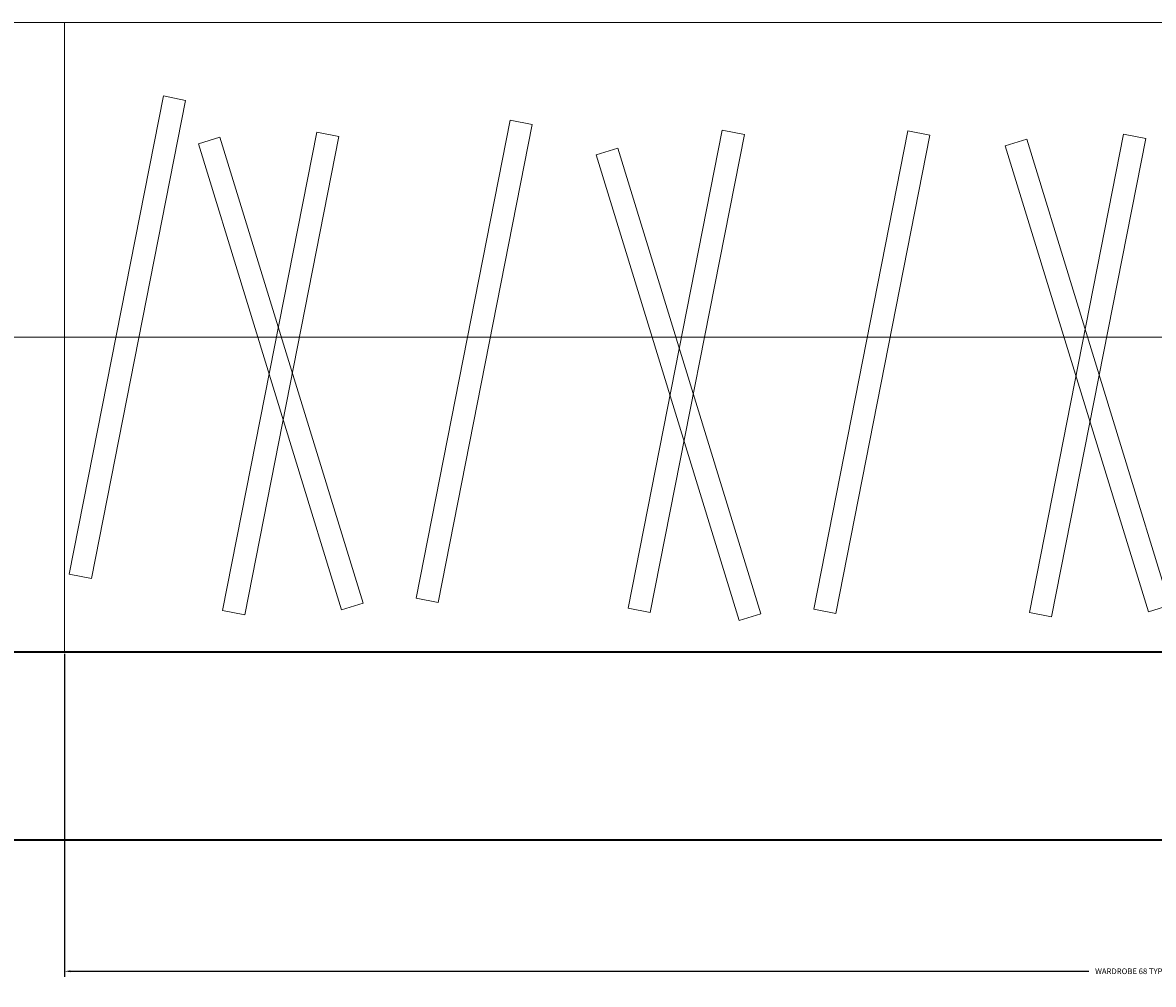
# Model space of a CAD drawing. Units: inches. Extents: x -61 to 1599, y -1316 to 257.
# Tile 180 of 204: x 1444 to 1480, y -788 to -757. Entities that reach past the tile are written whole.
import ezdxf

# ---------------------------------------------------------------- set-up
doc = ezdxf.new("R2010")
doc.units = ezdxf.units.IN
doc.header["$MEASUREMENT"] = 0
for name, color, linetype, lineweight in [('A-ANNO-DIMS', 2, 'Continuous', 18), ('A-FLOR-CASE', 8, 'Continuous', 18), ('WALLS', 4, 'Continuous', 35)]:
    doc.layers.add(name, color=color, linetype=linetype, lineweight=lineweight)
doc.styles.get("Standard").update_dxf_attribs({"font": 'arial.ttf'})
doc.dimstyles.get("Standard").update_dxf_attribs({"dimtxt": 0.18, "dimasz": 0.18, "dimexe": 0.18, "dimexo": 0.0625, "dimgap": 0.09, "dimtad": 0, "dimtih": 1, "dimtoh": 1, "dimdec": 0, "dimzin": 0, "dimdsep": 46, "dimlunit": 3, "dimtxsty": 'Standard', "dimcen": 0.09, "dimadec": 0, "dimazin": 0, "dimtfac": 1, "dimtdec": 0, "dimtofl": 0, "dimtmove": 0, "dimatfit": 3, "dimfxl": 1, "dimtolj": 1, "dimtzin": 0, "dimarcsym": 0})

# ---------------------------------------------------------------- blocks, each defined once
blk = doc.blocks.new('WARDROBE-HANGING')
blk.add_line((10.047, 0), (10.047, 68))
for points in [[(20.094, 0), (0, 0), (0, 68), (20.094, 68)], [(2.482, 67.852), (17.751, 64.849), (17.612, 64.142), (2.343, 67.146)], [(1.346, 59.162), (16.221, 63.731), (16.432, 63.043), (1.557, 58.474)], [(1.325, 62.957), (16.593, 59.954), (16.454, 59.247), (1.186, 62.251)], [(1.713, 56.784), (16.981, 53.781), (16.842, 53.074), (1.574, 56.078)], [(0.997, 46.467), (15.872, 51.036), (16.084, 50.348), (1.209, 45.779)], [(1.394, 50.014), (16.662, 47.011), (16.523, 46.305), (1.255, 49.308)], [(1.365, 44.09), (16.633, 41.086), (16.494, 40.38), (1.226, 43.383)], [(1.283, 33.408), (16.158, 37.977), (16.37, 37.289), (1.495, 32.72)], [(1.262, 37.203), (16.53, 34.2), (16.391, 33.493), (1.123, 36.497)], [(1.651, 31.03), (16.919, 28.027), (16.78, 27.32), (1.512, 30.324)], [(1.279, 21.299), (16.154, 25.868), (16.365, 25.18), (1.49, 20.611)], [(1.257, 25.094), (16.525, 22.091), (16.386, 21.384), (1.118, 24.388)], [(1.646, 18.921), (16.914, 15.918), (16.775, 15.211), (1.507, 18.215)], [(1.928, 9.892), (16.803, 14.461), (17.014, 13.773), (2.139, 9.203)], [(1.906, 13.687), (17.174, 10.684), (17.035, 9.977), (1.767, 12.981)], [(2.295, 7.514), (17.563, 4.511), (17.424, 3.804), (2.156, 6.808)], [(17.491, 1.962), (1.93, 1.962), (1.93, 2.682), (17.491, 2.682)]]:
    blk.add_lwpolyline(points, close=True)
blk = doc.blocks.new('WARDROBE-HANGING-4')
blk.add_line((68, 10.047), (0, 10.047))
for points in [[(68, 20.094), (68, 0), (0, 0), (0, 20.094)], [(0.148, 2.482), (3.151, 17.75), (3.858, 17.611), (0.854, 2.343)], [(11.216, 1.713), (14.219, 16.981), (14.925, 16.842), (11.922, 1.574)], [(58.108, 1.928), (53.539, 16.802), (54.227, 17.014), (58.796, 2.139)], [(54.313, 1.906), (57.316, 17.174), (58.023, 17.035), (55.019, 1.767)], [(17.985, 1.394), (20.989, 16.662), (21.695, 16.523), (18.692, 1.255)], [(23.91, 1.364), (26.914, 16.633), (27.62, 16.494), (24.617, 1.225)], [(36.97, 1.651), (39.973, 16.919), (40.68, 16.78), (37.676, 1.512)], [(49.079, 1.646), (52.082, 16.914), (52.788, 16.775), (49.785, 1.507)], [(8.838, 1.346), (4.269, 16.221), (4.957, 16.432), (9.526, 1.557)], [(5.043, 1.324), (8.046, 16.593), (8.753, 16.454), (5.749, 1.185)], [(34.592, 1.283), (30.023, 16.158), (30.711, 16.37), (35.28, 1.495)], [(30.797, 1.262), (33.8, 16.53), (34.507, 16.391), (31.503, 1.123)], [(46.701, 1.279), (42.132, 16.153), (42.82, 16.365), (47.389, 1.49)], [(42.906, 1.257), (45.909, 16.525), (46.616, 16.386), (43.612, 1.118)], [(21.533, 0.997), (16.964, 15.872), (17.652, 16.083), (22.221, 1.209)]]:
    blk.add_lwpolyline(points, close=True)
blk = doc.blocks.new('*D680')
at = {"layer": 'A-ANNO-DIMS', "color": 0, "lineweight": -2, "transparency": 16777216}
for p, q in [((1445.703, -777.232), (1445.703, -787.549)), ((1513.703, -777.232), (1513.703, -787.549)), ((1445.883, -787.369), (1478.396, -787.369)), ((1513.523, -787.369), (1481.01, -787.369))]:
    blk.add_line(p, q, dxfattribs=at)
at = {"layer": 'A-ANNO-DIMS', "color": 0, "transparency": 16777216}
for points in [[(1445.883, -787.339), (1445.883, -787.399), (1445.703, -787.369)], [(1513.523, -787.339), (1513.523, -787.399), (1513.703, -787.369)]]:
    blk.add_solid(points, dxfattribs=at)
at = {"layer": 'DEFPOINTS', "color": 0, "transparency": 16777216}
for p in [(1445.703, -777.169), (1513.703, -777.169), (1513.703, -787.369)]:
    blk.add_point(p, dxfattribs=at)
at = {"layer": 'A-ANNO-DIMS', "color": 0, "transparency": 16777216, "insert": (1479.703, -787.369), "char_height": 0.18, "attachment_point": 5}
blk.add_mtext('\\A1;WARDROBE 68 TYP.', dxfattribs=at)

msp = doc.modelspace()

# ---------------------------------------------------------------- linework, layer by layer
at = {"layer": 'WALLS'}
for p, q in [((1375.7028, -777.169), (1513.7028, -777.169)), ((1375.7028, -783.169), (1513.7028, -783.169))]:
    msp.add_line(p, q, dxfattribs=at)

# ---------------------------------------------------------------- block references
at = {"layer": 'A-FLOR-CASE', "rotation": 90.00000000000018}
msp.add_blockref('WARDROBE-HANGING', (1445.7029, -777.1692), dxfattribs=at)
at = {"layer": 'A-FLOR-CASE'}
msp.add_blockref('WARDROBE-HANGING-4', (1445.703, -777.1691), dxfattribs=at)

# ---------------------------------------------------------------- dimensions: what is measured, and where the dimension line sits
at = {"layer": 'A-ANNO-DIMS'}
dim = msp.add_linear_dim(base=(1513.7028, -787.369), p1=(1445.7028, -777.169), p2=(1513.7028, -777.169), text='WARDROBE <> TYP.', dimstyle='Standard', override={"dimdec": 0, "dimlfac": 1, "dimrnd": 0, "dimzin": 0, "dimdsep": 46, "dimlunit": 2}, dxfattribs=at)
dim.commit()
dim.dimension.update_dxf_attribs({"geometry": '*D680', "text_midpoint": (1479.7028, -787.369)})

doc.saveas('drawing.dxf')
